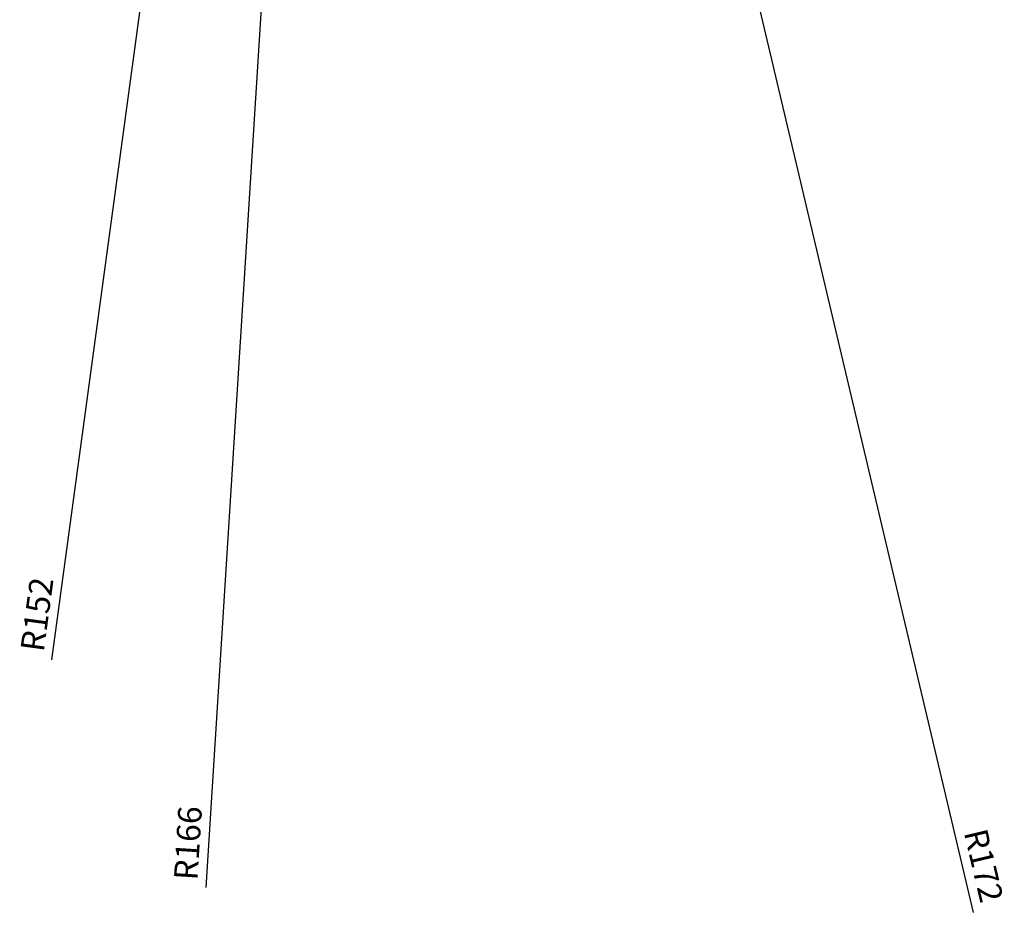
# Model space of a CAD drawing. Units: millimetres. Extents: x 2455 to 2735, y 1365 to 1648.
# Tile 1 of 3: x 2554 to 2658, y 1365 to 1460. Entities that reach past the tile are written whole.
import ezdxf

# ---------------------------------------------------------------- set-up
doc = ezdxf.new("R2010")
doc.units = ezdxf.units.MM
doc.layers.add('M-DIMS', color=2, linetype='Continuous', lineweight=25)
doc.styles.get("Standard").update_dxf_attribs({"font": 'arial.ttf'})
doc.dimstyles.new('ISO-25', dxfattribs={"dimtxt": 2.5, "dimasz": 2.5, "dimexe": 1.25, "dimexo": 0.625, "dimtad": 1, "dimdec": 0, "dimtxsty": 'Standard', "dimcen": 2.5, "dimadec": 0, "dimazin": 0, "dimtfac": 1, "dimtdec": 0, "dimtmove": 0, "dimatfit": 3, "dimfxl": 1, "dimarcsym": 0})

# ---------------------------------------------------------------- blocks, each defined once
blk = doc.blocks.new('*D40')
at = {"layer": 'Defpoints', "color": 0, "transparency": 16777216}
for p in [(2590.42, 1637.21), (2629.97, 1469.82)]:
    blk.add_point(p, dxfattribs=at)
at = {"layer": 'M-DIMS', "color": 0, "lineweight": -2, "transparency": 16777216}
for p, q in [((2590.42, 1637.21), (2629.97, 1469.82)), ((2654.75, 1364.93), (2630.55, 1467.38))]:
    blk.add_line(p, q, dxfattribs=at)
at = {"layer": 'M-DIMS', "color": 0, "transparency": 16777216}
blk.add_solid([(2630.95, 1467.48), (2630.14, 1467.29), (2629.97, 1469.82)], dxfattribs=at)
at = {"layer": 'M-DIMS', "color": 0, "transparency": 16777216, "insert": (2655.53, 1369.81), "char_height": 2.5, "attachment_point": 5, "rotation": 283.2931}
blk.add_mtext('R172', dxfattribs=at)
blk = doc.blocks.new('*D41')
at = {"layer": 'Defpoints', "color": 0, "transparency": 16777216}
for p in [(2590.42, 1637.21), (2569.99, 1486.59)]:
    blk.add_point(p, dxfattribs=at)
at = {"layer": 'M-DIMS', "color": 0, "lineweight": -2, "transparency": 16777216}
for p, q in [((2590.42, 1637.21), (2569.99, 1486.59)), ((2557.12, 1391.69), (2569.66, 1484.11))]:
    blk.add_line(p, q, dxfattribs=at)
at = {"layer": 'M-DIMS', "color": 0, "transparency": 16777216}
blk.add_solid([(2569.24, 1484.17), (2570.07, 1484.05), (2569.99, 1486.59)], dxfattribs=at)
at = {"layer": 'M-DIMS', "color": 0, "transparency": 16777216, "insert": (2555.85, 1396.47), "char_height": 2.5, "attachment_point": 5, "rotation": 82.2752}
blk.add_mtext('R152', dxfattribs=at)
blk = doc.blocks.new('*D42')
at = {"layer": 'Defpoints', "color": 0, "transparency": 16777216}
for p in [(2590.42, 1637.21), (2580, 1471.54)]:
    blk.add_point(p, dxfattribs=at)
at = {"layer": 'M-DIMS', "color": 0, "lineweight": -2, "transparency": 16777216}
for p, q in [((2590.42, 1637.21), (2580, 1471.54)), ((2573.46, 1367.56), (2579.84, 1469.04))]:
    blk.add_line(p, q, dxfattribs=at)
at = {"layer": 'M-DIMS', "color": 0, "transparency": 16777216}
blk.add_solid([(2579.43, 1469.07), (2580.26, 1469.01), (2580, 1471.54)], dxfattribs=at)
at = {"layer": 'M-DIMS', "color": 0, "transparency": 16777216, "insert": (2571.85, 1372.25), "char_height": 2.5, "attachment_point": 5, "rotation": 86.3994}
blk.add_mtext('R166', dxfattribs=at)

msp = doc.modelspace()

# ---------------------------------------------------------------- dimensions: what is measured, and where the dimension line sits
at = {"layer": 'M-DIMS'}
for mpoint, picture, middle in [((2569.9929, 1486.5875), '*D41', (2557.7342, 1396.2151)), ((2579.9991, 1471.5357), '*D42', (2573.7441, 1372.1323)), ((2629.9725, 1469.8165), '*D40', (2653.7015, 1369.3816))]:
    dim = msp.add_radius_dim(center=(2590.424, 1637.2081), mpoint=mpoint, dimstyle='ISO-25', override={"dimdec": 0, "dimlfac": 1, "dimrnd": 0, "dimzin": 0, "dimdsep": 46, "dimlunit": 2}, dxfattribs=at)
    dim.commit()
    dim.dimension.update_dxf_attribs({"geometry": picture, "text_midpoint": middle, "dimtype": 164})

doc.saveas('drawing.dxf')
